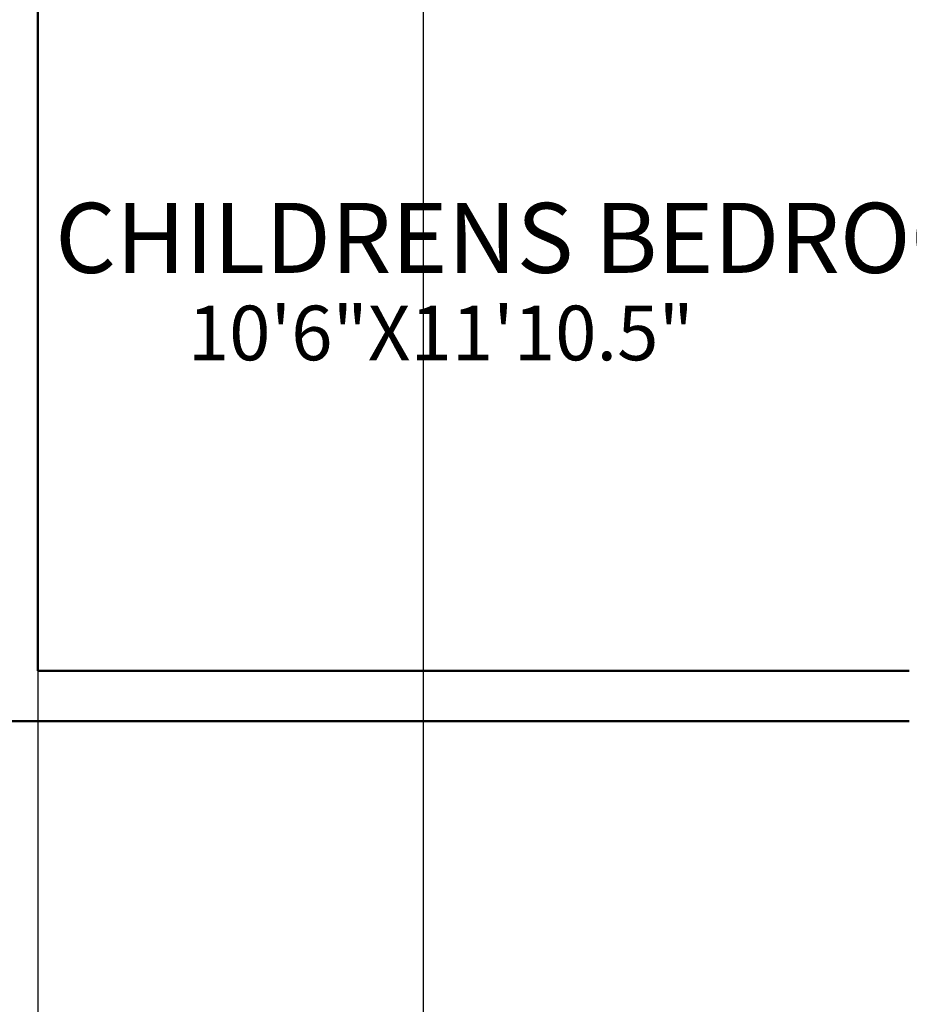
# Model space of a CAD drawing. Units: inches. Extents: x 7359 to 7979, y 33027 to 34263.
# Tile 14 of 32: x 7612 to 7691, y 33446 to 33534. Entities that reach past the tile are written whole.
import ezdxf

# ---------------------------------------------------------------- set-up
doc = ezdxf.new("R2010")
doc.units = ezdxf.units.IN
for name, color, linetype, lineweight in [('A-ANNO-DIMS', 2, 'Continuous', 18), ('A-AREA-IDEN', 7, 'Continuous', 18), ('A-WALL', 7, 'Continuous', 50)]:
    doc.layers.add(name, color=color, linetype=linetype, lineweight=lineweight)
doc.styles.get("Standard").update_dxf_attribs({"font": 'arial.ttf'})
doc.dimstyles.get("Standard").update_dxf_attribs({"dimtxt": 0.18, "dimasz": 0.18, "dimexe": 0.18, "dimexo": 0.0625, "dimgap": 0.09, "dimtad": 0, "dimtih": 1, "dimtoh": 1, "dimdec": 4, "dimzin": 0, "dimdsep": 46, "dimtxsty": 'Standard', "dimcen": 0.09, "dimadec": 0, "dimazin": 0, "dimtfac": 1, "dimtdec": 4, "dimtofl": 0, "dimtmove": 0, "dimatfit": 3, "dimfxl": 1, "dimtolj": 1, "dimtzin": 0, "dimarcsym": 0})

# ---------------------------------------------------------------- blocks, each defined once
blk = doc.blocks.new('*D73')
at = {"layer": 'A-ANNO-DIMS', "color": 0, "lineweight": -2, "transparency": 16777216}
for p, q in [((7613.227, 33618.1), (7613.227, 33027.177)), ((7647.706, 33618.1), (7647.706, 33027.177)), ((7613.407, 33027.357), (7630.073, 33027.357)), ((7647.526, 33027.357), (7630.86, 33027.357))]:
    blk.add_line(p, q, dxfattribs=at)
at = {"layer": 'A-ANNO-DIMS', "color": 0, "transparency": 16777216}
for points in [[(7613.407, 33027.387), (7613.407, 33027.327), (7613.227, 33027.357)], [(7647.526, 33027.387), (7647.526, 33027.327), (7647.706, 33027.357)]]:
    blk.add_solid(points, dxfattribs=at)
at = {"layer": 'Defpoints', "color": 0, "transparency": 16777216}
for p in [(7613.227, 33618.162), (7647.706, 33618.162), (7647.706, 33027.357)]:
    blk.add_point(p, dxfattribs=at)
at = {"layer": 'A-ANNO-DIMS', "color": 0, "transparency": 16777216, "insert": (7630.466, 33027.357), "char_height": 0.18, "attachment_point": 5}
blk.add_mtext('\\A1;34.48', dxfattribs=at)

msp = doc.modelspace()

# ---------------------------------------------------------------- linework, layer by layer
at = {"layer": 'A-WALL'}
for p, q in [((7613.2266, 33618.1623), (7613.2266, 33475.6623)), ((7613.2266, 33475.6623), (7691.2266, 33475.6623)), ((7602.7266, 33471.1623), (7691.2266, 33471.1623))]:
    msp.add_line(p, q, dxfattribs=at)

# ---------------------------------------------------------------- texts
at = {"layer": 'A-AREA-IDEN'}
for s, height, p in [('CHILDRENS BEDROOM', 6.259411, (7614.7656, 33511.2719)), ('10\'6"X11\'10.5"', 4.885549, (7626.6414, 33503.454))]:
    msp.add_text(s, height=height, dxfattribs=at).set_placement(p)

# ---------------------------------------------------------------- dimensions: what is measured, and where the dimension line sits
at = {"layer": 'A-ANNO-DIMS'}
dim = msp.add_linear_dim(base=(7647.7062, 33027.3568), p1=(7613.2266, 33618.1623), p2=(7647.7062, 33618.1623), dimstyle='Standard', override={"dimdec": 2, "dimlfac": 1, "dimrnd": 0, "dimzin": 0, "dimdsep": 46, "dimlunit": 2}, dxfattribs=at)
dim.commit()
dim.dimension.update_dxf_attribs({"geometry": '*D73', "text_midpoint": (7630.4664, 33027.3568)})

doc.saveas('drawing.dxf')
